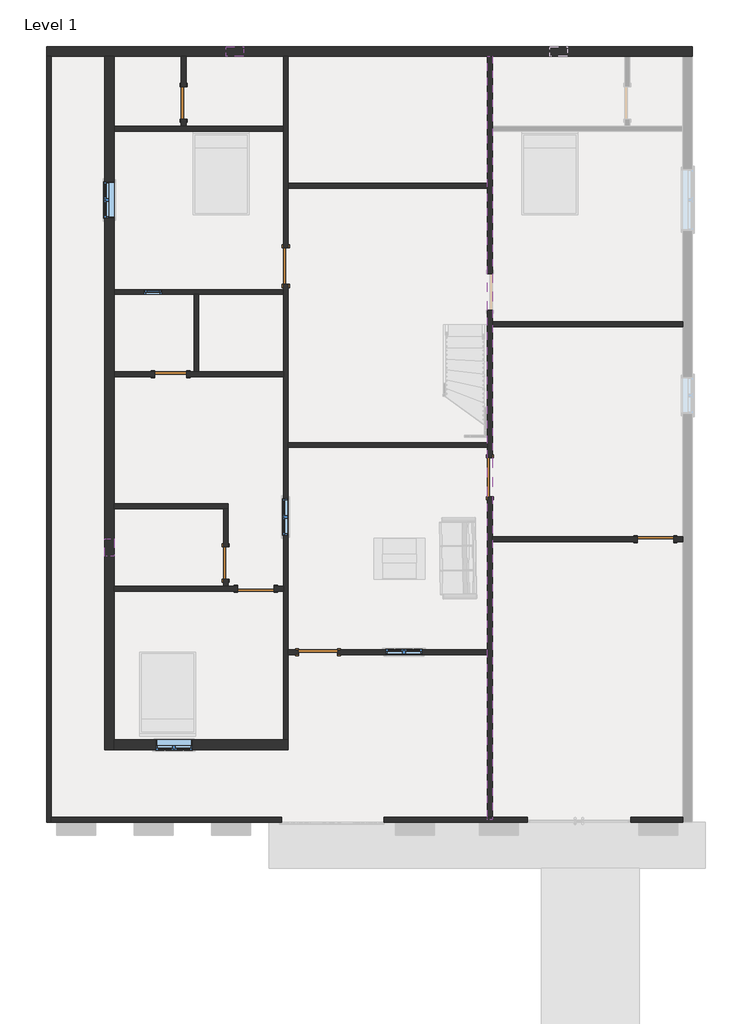
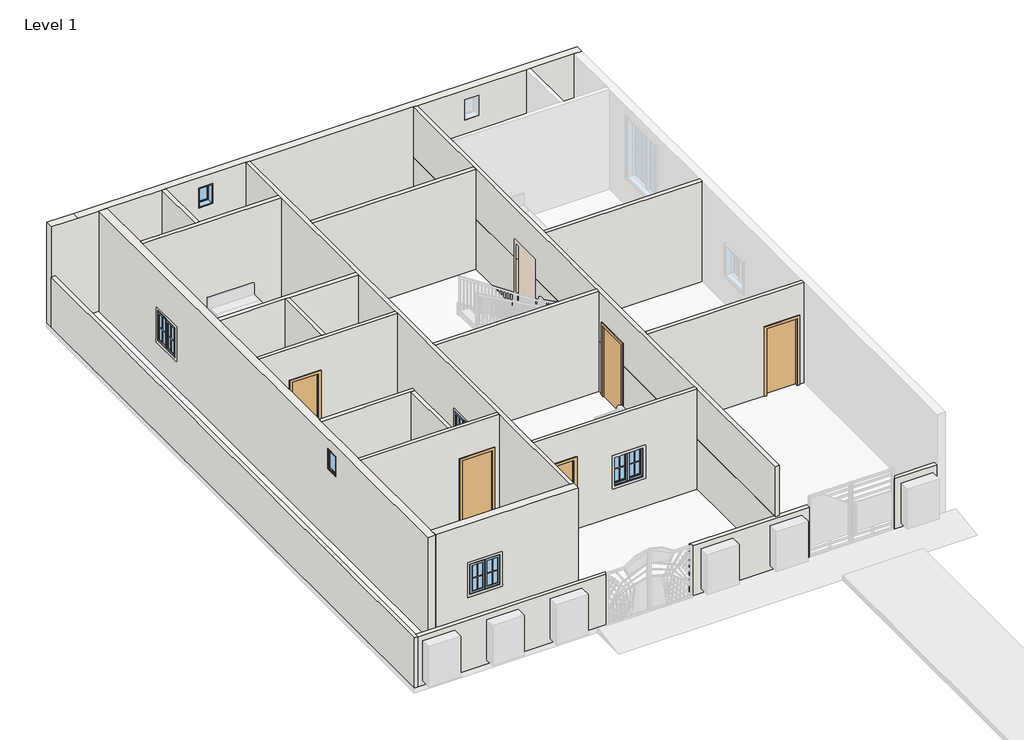
# One storey, part 1 of 3: 23 walls, 8 doors, 7 windows.
"""IFC4 building model written with IfcOpenShell, lengths in millimetres."""

from ifc_helpers import new_model, si_unit, frame, origin, origin_with_axes, place, context, project, spatial, polyline, outline, extrude, faceted_brep, transform, mapped, element, save
from components import door_f2b275c1, door_d8f5dbb5, door_825b8444, door_c29894e6, door_305aa2a5, window_aa618e30, window_a10b4202, window_339605e1, window_a598f463

model = new_model("IFC4")

# Units and contexts
model_context = context("Model", 3, world=origin())
ifc_project = project(units=[si_unit("LENGTHUNIT", "METRE", prefix="MILLI")], contexts=[model_context])

# Site, building, storey
site = spatial("IfcSite", under=ifc_project)
building = spatial("IfcBuilding", under=site)
storey = spatial("IfcBuildingStorey", under=building, Name="Level 1", Elevation=0.0)

# Doors
placement = place(None, origin())
door_shape = door_f2b275c1(model_context)
element("IfcDoor", 1, ObjectType="Single-Flush : 30\" x 80\"", at=placement, inside=storey, context=model_context, shape_type="MappedRepresentation", body=[
    mapped(door_shape, transform((-5639.8561469, 9100.7522623, 0.0), x_axis=(0.0, -1.0, 0.0), y_axis=(1.0, 0.0, 0.0), z_axis=(0.0, 0.0, 1.0))),
])
element("IfcDoor", 2, ObjectType="Single-Flush : 30\" x 80\"", at=placement, inside=storey, context=model_context, shape_type="MappedRepresentation", body=[
    mapped(door_shape, transform((-4646.033646, -1745.0477377, 0.0), x_axis=(0.0, -1.0, 0.0), y_axis=(1.0, 0.0, 0.0), z_axis=(0.0, 0.0, 1.0))),
])
door_2_shape = door_d8f5dbb5(model_context)
element("IfcDoor", 3, ObjectType="Single-Flush : 30\" x 80\"", at=placement, inside=storey, context=model_context, shape_type="MappedRepresentation", body=[
    mapped(door_2_shape, transform((-5947.8915084, 2699.9522623, 0.0), x_axis=(1.0, 0.0, 0.0), y_axis=(0.0, 1.0, 0.0), z_axis=(0.0, 0.0, 1.0))),
])
door_3_shape = door_825b8444(model_context)
element("IfcDoor", 4, ObjectType="Single-Flush : 34\" x 80\"", at=placement, inside=storey, context=model_context, shape_type="MappedRepresentation", body=[
    mapped(door_3_shape, transform((-3230.0915084, 5252.6522623, 0.0), x_axis=(0.0, -1.0, 0.0), y_axis=(1.0, 0.0, 0.0), z_axis=(0.0, 0.0, 1.0))),
])
element("IfcDoor", 5, ObjectType="Single-Flush : 34\" x 80\"", at=placement, inside=storey, context=model_context, shape_type="MappedRepresentation", body=[
    mapped(door_3_shape, transform((-3938.0625772, -2354.6477377, 0.0), x_axis=(1.0, 0.0, 0.0), y_axis=(0.0, 1.0, 0.0), z_axis=(0.0, 0.0, 1.0))),
])
door_4_shape = door_c29894e6(model_context)
element("IfcDoor", 6, ObjectType="Single-Flush : 34\" x 80\"", at=placement, inside=storey, context=model_context, shape_type="MappedRepresentation", body=[
    mapped(door_4_shape, transform((5488.4584916, -1186.2477377, 0.0), x_axis=(1.0, 0.0, 0.0), y_axis=(0.0, 1.0, 0.0), z_axis=(0.0, 0.0, 1.0))),
])
door_5_shape = door_305aa2a5(model_context)
element("IfcDoor", 7, ObjectType="Single-Flush : 36\" x 84\"", at=placement, inside=storey, context=model_context, shape_type="MappedRepresentation", body=[
    mapped(door_5_shape, transform((1583.2084916, 274.2522623, 0.0), x_axis=(0.0, -1.0, 0.0), y_axis=(1.0, 0.0, 0.0), z_axis=(0.0, 0.0, 1.0))),
])
element("IfcDoor", 8, ObjectType="Single-Flush : 36\" x 84\"", at=placement, inside=storey, context=model_context, shape_type="MappedRepresentation", body=[
    mapped(door_5_shape, transform((-2468.0915084, -3853.2477377, 0.0), x_axis=(-1.0, 0.0, 0.0), y_axis=(0.0, -1.0, 0.0), z_axis=(0.0, 0.0, 1.0))),
])

# Walls
element("IfcWall", 9, ObjectType="9\"", at=placement, inside=storey, context=model_context, shape_type="Brep", body=[
    faceted_brep([(-8875.2415084, 10199.3022623, 0.0), (-8760.9415084, 10199.3022623, 0.0), (-7503.6415084, 10199.3022623, 0.0), (-7275.0415084, 10199.3022623, 0.0), (-5697.0061469, 10199.3022623, 0.0), (-5582.7061469, 10199.3022623, 0.0), (-3287.2415084, 10199.3022623, 0.0), (-3172.9415084, 10199.3022623, 0.0), (1526.0584916, 10199.3022623, 0.0), (1640.3584916, 10199.3022623, 0.0), (4770.1866507, 10199.3022623, 0.0), (4884.4866507, 10199.3022623, 0.0), (6136.1584916, 10199.3022623, 0.0), (6364.7584916, 10199.3022623, 0.0), (6364.7584916, 10199.3022623, 3048.0), (6136.1584916, 10199.3022623, 3048.0), (4884.4866507, 10199.3022623, 3048.0), (4770.1866507, 10199.3022623, 3048.0), (1640.3584916, 10199.3022623, 3048.0), (1526.0584916, 10199.3022623, 3048.0), (-3172.9415084, 10199.3022623, 3048.0), (-3287.2415084, 10199.3022623, 3048.0), (-5582.7061469, 10199.3022623, 3048.0), (-5697.0061469, 10199.3022623, 3048.0), (-7275.0415084, 10199.3022623, 3048.0), (-7503.6415084, 10199.3022623, 3048.0), (-8113.2415084, 10199.3022623, 3048.0), (-8875.2415084, 10199.3022623, 3048.0), (-8875.2415084, 10199.3022623, 1524.0), (-4231.7738276, 10199.3022623, 2743.2), (-4231.7738276, 10199.3022623, 2133.6), (-4638.1738276, 10199.3022623, 2133.6), (-4638.1738276, 10199.3022623, 2743.2), (3408.4725711, 10199.3022623, 2743.2), (3408.4725711, 10199.3022623, 2133.6), (3002.0725711, 10199.3022623, 2133.6), (3002.0725711, 10199.3022623, 2743.2), (-8875.2415084, 10427.9022623, 0.0), (-8875.2415084, 10427.9022623, 3048.0), (-8113.2415084, 10427.9022623, 3048.0), (6364.7584916, 10427.9022623, 3048.0), (6364.7584916, 10427.9022623, 0.0), (-4231.7738276, 10427.9022623, 2743.2), (-4638.1738276, 10427.9022623, 2743.2), (-4638.1738276, 10427.9022623, 2133.6), (-4231.7738276, 10427.9022623, 2133.6), (3408.4725711, 10427.9022623, 2743.2), (3002.0725711, 10427.9022623, 2743.2), (3002.0725711, 10427.9022623, 2133.6), (3408.4725711, 10427.9022623, 2133.6)], [[[0, 1, 2, 3, 4, 5, 6, 7, 8, 9, 10, 11, 12, 13, 14, 15, 16, 17, 18, 19, 20, 21, 22, 23, 24, 25, 26, 27, 28], [29, 30, 31, 32], [33, 34, 35, 36]], [[37, 38, 39, 40, 41], [42, 43, 44, 45], [46, 47, 48, 49]], [[13, 12, 11, 10, 9, 8, 7, 6, 5, 4, 3, 2, 1, 0, 37, 41]], [[14, 13, 41, 40]], [[0, 28, 27, 38, 37]], [[30, 29, 42, 45]], [[31, 30, 45, 44]], [[32, 31, 44, 43]], [[29, 32, 43, 42]], [[34, 33, 46, 49]], [[35, 34, 49, 48]], [[36, 35, 48, 47]], [[33, 36, 47, 46]], [[27, 26, 39, 38]], [[26, 25, 24, 23, 22, 21, 20, 19, 18, 17, 16, 15, 14, 40, 39]]]),
])
element("IfcWall", 10, ObjectType="9\"", at=placement, inside=storey, context=model_context, shape_type="Brep", body=[
    faceted_brep([(-7503.6415084, 10199.3022623, 0.0), (-7503.6415084, -6145.5977377, 0.0), (-7503.6415084, -6145.5977377, 3048.0), (-7503.6415084, 10199.3022623, 3048.0), (-7503.6415084, -1179.8977377, 2743.2), (-7503.6415084, -1586.2977377, 2743.2), (-7503.6415084, -1586.2977377, 2133.6), (-7503.6415084, -1179.8977377, 2133.6), (-7503.6415084, 7246.5522623, 1828.8), (-7503.6415084, 6382.9522623, 1828.8), (-7503.6415084, 6382.9522623, 914.4), (-7503.6415084, 7246.5522623, 914.4), (-7275.0415084, 10199.3022623, 0.0), (-7275.0415084, 10199.3022623, 3048.0), (-7275.0415084, 8548.3022623, 3048.0), (-7275.0415084, 8434.0022623, 3048.0), (-7275.0415084, 4700.2022623, 3048.0), (-7275.0415084, 4585.9022623, 3048.0), (-7275.0415084, 2757.1022623, 3048.0), (-7275.0415084, 2642.8022623, 3048.0), (-7275.0415084, -354.3977377, 3048.0), (-7275.0415084, -468.6977377, 3048.0), (-7275.0415084, -2297.4977377, 3048.0), (-7275.0415084, -2411.7977377, 3048.0), (-7275.0415084, -5916.9977377, 3048.0), (-7275.0415084, -6145.5977377, 3048.0), (-7275.0415084, -6145.5977377, 0.0), (-7275.0415084, -5916.9977377, 0.0), (-7275.0415084, -2411.7977377, 0.0), (-7275.0415084, -2297.4977377, 0.0), (-7275.0415084, -468.6977377, 0.0), (-7275.0415084, -354.3977377, 0.0), (-7275.0415084, 2642.8022623, 0.0), (-7275.0415084, 2757.1022623, 0.0), (-7275.0415084, 4585.9022623, 0.0), (-7275.0415084, 4700.2022623, 0.0), (-7275.0415084, 8434.0022623, 0.0), (-7275.0415084, 8548.3022623, 0.0), (-7275.0415084, -1179.8977377, 2743.2), (-7275.0415084, -1179.8977377, 2133.6), (-7275.0415084, -1586.2977377, 2133.6), (-7275.0415084, -1586.2977377, 2743.2), (-7275.0415084, 7246.5522623, 1828.8), (-7275.0415084, 7246.5522623, 914.4), (-7275.0415084, 6382.9522623, 914.4), (-7275.0415084, 6382.9522623, 1828.8)], [[[0, 1, 2, 3], [4, 5, 6, 7], [8, 9, 10, 11]], [[12, 13, 14, 15, 16, 17, 18, 19, 20, 21, 22, 23, 24, 25, 26, 27, 28, 29, 30, 31, 32, 33, 34, 35, 36, 37], [38, 39, 40, 41], [42, 43, 44, 45]], [[1, 0, 12, 37, 36, 35, 34, 33, 32, 31, 30, 29, 28, 27, 26]], [[0, 3, 13, 12]], [[2, 1, 26, 25]], [[39, 38, 4, 7]], [[40, 39, 7, 6]], [[41, 40, 6, 5]], [[38, 41, 5, 4]], [[43, 42, 8, 11]], [[44, 43, 11, 10]], [[45, 44, 10, 9]], [[42, 45, 9, 8]], [[3, 2, 25, 24, 23, 22, 21, 20, 19, 18, 17, 16, 15, 14, 13]]]),
])
element("IfcWall", 11, ObjectType="9\"", at=placement, inside=storey, context=model_context, shape_type="Brep", body=[
    faceted_brep([(-7275.0415084, -6145.5977377, 0.0), (-3172.9415084, -6145.5977377, 0.0), (-3172.9415084, -6145.5977377, 3048.0), (-7275.0415084, -6145.5977377, 3048.0), (-6297.1415084, -6145.5977377, 1828.8), (-5433.5415084, -6145.5977377, 1828.8), (-5433.5415084, -6145.5977377, 914.4), (-6297.1415084, -6145.5977377, 914.4), (-7275.0415084, -5916.9977377, 0.0), (-7275.0415084, -5916.9977377, 3048.0), (-3287.2415084, -5916.9977377, 3048.0), (-3172.9415084, -5916.9977377, 3048.0), (-3172.9415084, -5916.9977377, 0.0), (-3287.2415084, -5916.9977377, 0.0), (-6297.1415084, -5916.9977377, 1828.8), (-6297.1415084, -5916.9977377, 914.4), (-5433.5415084, -5916.9977377, 914.4), (-5433.5415084, -5916.9977377, 1828.8)], [[[0, 1, 2, 3], [4, 5, 6, 7]], [[8, 9, 10, 11, 12, 13], [14, 15, 16, 17]], [[1, 0, 8, 13, 12]], [[0, 3, 9, 8]], [[2, 1, 12, 11]], [[15, 14, 4, 7]], [[16, 15, 7, 6]], [[17, 16, 6, 5]], [[14, 17, 5, 4]], [[3, 2, 11, 10, 9]]]),
])
element("IfcWall", 12, ObjectType="WALL4.5\"", at=placement, inside=storey, context=model_context, shape_type="Brep", body=[
    faceted_brep([(-8875.2415084, 10199.3022623, 0.0), (-8875.2415084, -7860.0977377, 0.0), (-8875.2415084, -7860.0977377, 1524.0), (-8875.2415084, 10199.3022623, 1524.0), (-8760.9415084, 10199.3022623, 0.0), (-8760.9415084, 10199.3022623, 1524.0), (-8760.9415084, -7745.7977377, 1524.0), (-8760.9415084, -7860.0977377, 1524.0), (-8760.9415084, -7860.0977377, 0.0), (-8760.9415084, -7745.7977377, 0.0)], [[[0, 1, 2, 3]], [[4, 5, 6, 7, 8, 9]], [[1, 0, 4, 9, 8]], [[3, 2, 7, 6, 5]], [[0, 3, 5, 4]], [[2, 1, 8, 7]]]),
])
element("IfcWall", 13, ObjectType="WALL4.5\"", at=placement, inside=storey, context=model_context, shape_type="SweptSolid", body=[
    extrude(outline(polyline([(-3331.6915084, -7860.0977377), (-8760.9415084, -7860.0977377), (-8760.9415084, -7745.7977377), (-3331.6915084, -7745.7977377), (-3331.6915084, -7860.0977377)])), origin_with_axes(), (0.0, 0.0, 1.0), 1524.0),
])
element("IfcWall", 14, ObjectType="WALL4.5\"", at=placement, inside=storey, context=model_context, shape_type="Brep", body=[
    faceted_brep([(-7275.0415084, 8434.0022623, 0.0), (-3287.2415084, 8434.0022623, 0.0), (-3287.2415084, 8434.0022623, 3048.0), (-7275.0415084, 8434.0022623, 3048.0), (-7275.0415084, 8548.3022623, 0.0), (-7275.0415084, 8548.3022623, 3048.0), (-5697.0061469, 8548.3022623, 3048.0), (-5582.7061469, 8548.3022623, 3048.0), (-3287.2415084, 8548.3022623, 3048.0), (-3287.2415084, 8548.3022623, 0.0), (-5582.7061469, 8548.3022623, 0.0), (-5697.0061469, 8548.3022623, 0.0)], [[[0, 1, 2, 3]], [[4, 5, 6, 7, 8, 9, 10, 11]], [[1, 0, 4, 11, 10, 9]], [[0, 3, 5, 4]], [[2, 1, 9, 8]], [[3, 2, 8, 7, 6, 5]]]),
])
element("IfcWall", 15, ObjectType="WALL4.5\"", at=placement, inside=storey, context=model_context, shape_type="SweptSolid", body=[
    extrude(outline(polyline([(8719.7522623, 2032.0), (8719.7522623, 0.0), (8548.3022623, 0.0), (8548.3022623, 3048.0), (10199.3022623, 3048.0), (10199.3022623, 0.0), (9481.7522623, 0.0), (9481.7522623, 2032.0), (8719.7522623, 2032.0)])), frame((-5697.0061469, 0.0, 0.0), z_axis=(1.0, 0.0, 0.0), x_axis=(0.0, 1.0, 0.0)), (0.0, 0.0, 1.0), 114.3),
])
element("IfcWall", 16, ObjectType="WALL4.5\"", at=placement, inside=storey, context=model_context, shape_type="Brep", body=[
    faceted_brep([(-3287.2415084, 4820.8522623, 2032.0), (-3287.2415084, 4820.8522623, 0.0), (-3287.2415084, 4700.2022623, 0.0), (-3287.2415084, 4585.9022623, 0.0), (-3287.2415084, 2757.1022623, 0.0), (-3287.2415084, 2642.8022623, 0.0), (-3287.2415084, -2297.4977377, 0.0), (-3287.2415084, -2411.7977377, 0.0), (-3287.2415084, -5916.9977377, 0.0), (-3287.2415084, -5916.9977377, 3048.0), (-3287.2415084, -2411.7977377, 3048.0), (-3287.2415084, -2297.4977377, 3048.0), (-3287.2415084, 2642.8022623, 3048.0), (-3287.2415084, 2757.1022623, 3048.0), (-3287.2415084, 4585.9022623, 3048.0), (-3287.2415084, 4700.2022623, 3048.0), (-3287.2415084, 8434.0022623, 3048.0), (-3287.2415084, 8548.3022623, 3048.0), (-3287.2415084, 10199.3022623, 3048.0), (-3287.2415084, 10199.3022623, 0.0), (-3287.2415084, 8548.3022623, 0.0), (-3287.2415084, 8434.0022623, 0.0), (-3287.2415084, 5684.4522623, 0.0), (-3287.2415084, 5684.4522623, 2032.0), (-3287.2415084, -227.3977377, 1828.8), (-3287.2415084, -1090.9977377, 1828.8), (-3287.2415084, -1090.9977377, 914.4), (-3287.2415084, -227.3977377, 914.4), (-3172.9415084, -5916.9977377, 0.0), (-3172.9415084, -3910.3977377, 0.0), (-3172.9415084, -3796.0977377, 0.0), (-3172.9415084, 979.1022623, 0.0), (-3172.9415084, 1093.4022623, 0.0), (-3172.9415084, 4820.8522623, 0.0), (-3172.9415084, 4820.8522623, 2032.0), (-3172.9415084, 5684.4522623, 2032.0), (-3172.9415084, 5684.4522623, 0.0), (-3172.9415084, 7087.8022623, 0.0), (-3172.9415084, 7202.1022623, 0.0), (-3172.9415084, 10199.3022623, 0.0), (-3172.9415084, 10199.3022623, 3048.0), (-3172.9415084, 7202.1022623, 3048.0), (-3172.9415084, 7087.8022623, 3048.0), (-3172.9415084, 1093.4022623, 3048.0), (-3172.9415084, 979.1022623, 3048.0), (-3172.9415084, -3796.0977377, 3048.0), (-3172.9415084, -3910.3977377, 3048.0), (-3172.9415084, -5916.9977377, 3048.0), (-3172.9415084, -227.3977377, 1828.8), (-3172.9415084, -227.3977377, 914.4), (-3172.9415084, -1090.9977377, 914.4), (-3172.9415084, -1090.9977377, 1828.8)], [[[0, 1, 2, 3, 4, 5, 6, 7, 8, 9, 10, 11, 12, 13, 14, 15, 16, 17, 18, 19, 20, 21, 22, 23], [24, 25, 26, 27]], [[28, 29, 30, 31, 32, 33, 34, 35, 36, 37, 38, 39, 40, 41, 42, 43, 44, 45, 46, 47], [48, 49, 50, 51]], [[22, 21, 20, 19, 39, 38, 37, 36]], [[8, 7, 6, 5, 4, 3, 2, 1, 33, 32, 31, 30, 29, 28]], [[9, 8, 28, 47]], [[19, 18, 40, 39]], [[34, 33, 1, 0]], [[35, 34, 0, 23]], [[36, 35, 23, 22]], [[49, 48, 24, 27]], [[50, 49, 27, 26]], [[51, 50, 26, 25]], [[48, 51, 25, 24]], [[18, 17, 16, 15, 14, 13, 12, 11, 10, 9, 47, 46, 45, 44, 43, 42, 41, 40]]]),
])
element("IfcWall", 17, ObjectType="WALL4.5\"", at=placement, inside=storey, context=model_context, shape_type="Brep", body=[
    faceted_brep([(-7275.0415084, 4585.9022623, 0.0), (-5395.4415084, 4585.9022623, 0.0), (-5281.1415084, 4585.9022623, 0.0), (-3287.2415084, 4585.9022623, 0.0), (-3287.2415084, 4585.9022623, 3048.0), (-5281.1415084, 4585.9022623, 3048.0), (-5395.4415084, 4585.9022623, 3048.0), (-7275.0415084, 4585.9022623, 3048.0), (-6160.6165084, 4585.9022623, 1524.0), (-6160.6165084, 4585.9022623, 914.4), (-6567.0165084, 4585.9022623, 914.4), (-6567.0165084, 4585.9022623, 1524.0), (-7275.0415084, 4700.2022623, 0.0), (-7275.0415084, 4700.2022623, 3048.0), (-3287.2415084, 4700.2022623, 3048.0), (-3287.2415084, 4700.2022623, 0.0), (-6160.6165084, 4700.2022623, 1524.0), (-6567.0165084, 4700.2022623, 1524.0), (-6567.0165084, 4700.2022623, 914.4), (-6160.6165084, 4700.2022623, 914.4)], [[[0, 1, 2, 3, 4, 5, 6, 7], [8, 9, 10, 11]], [[12, 13, 14, 15], [16, 17, 18, 19]], [[3, 2, 1, 0, 12, 15]], [[0, 7, 13, 12]], [[4, 3, 15, 14]], [[9, 8, 16, 19]], [[10, 9, 19, 18]], [[11, 10, 18, 17]], [[8, 11, 17, 16]], [[7, 6, 5, 4, 14, 13]]]),
])
element("IfcWall", 18, ObjectType="WALL4.5\"", at=placement, inside=storey, context=model_context, shape_type="SweptSolid", body=[
    extrude(outline(polyline([(-5395.4415084, 2757.1022623), (-5395.4415084, 4585.9022623), (-5281.1415084, 4585.9022623), (-5281.1415084, 2757.1022623), (-5395.4415084, 2757.1022623)])), origin_with_axes(), (0.0, 0.0, 1.0), 3048.0),
])
element("IfcWall", 19, ObjectType="WALL4.5\"", at=placement, inside=storey, context=model_context, shape_type="Brep", body=[
    faceted_brep([(-5566.8915084, 2642.8022623, 2032.0), (-5566.8915084, 2642.8022623, 0.0), (-3287.2415084, 2642.8022623, 0.0), (-3287.2415084, 2642.8022623, 3048.0), (-7275.0415084, 2642.8022623, 3048.0), (-7275.0415084, 2642.8022623, 0.0), (-6328.8915084, 2642.8022623, 0.0), (-6328.8915084, 2642.8022623, 2032.0), (-3287.2415084, 2757.1022623, 0.0), (-5281.1415084, 2757.1022623, 0.0), (-5395.4415084, 2757.1022623, 0.0), (-5566.8915084, 2757.1022623, 0.0), (-5566.8915084, 2757.1022623, 2032.0), (-6328.8915084, 2757.1022623, 2032.0), (-6328.8915084, 2757.1022623, 0.0), (-7275.0415084, 2757.1022623, 0.0), (-7275.0415084, 2757.1022623, 3048.0), (-5395.4415084, 2757.1022623, 3048.0), (-5281.1415084, 2757.1022623, 3048.0), (-3287.2415084, 2757.1022623, 3048.0)], [[[0, 1, 2, 3, 4, 5, 6, 7]], [[8, 9, 10, 11, 12, 13, 14, 15, 16, 17, 18, 19]], [[6, 5, 15, 14]], [[2, 1, 11, 10, 9, 8]], [[5, 4, 16, 15]], [[3, 2, 8, 19]], [[12, 11, 1, 0]], [[13, 12, 0, 7]], [[14, 13, 7, 6]], [[4, 3, 19, 18, 17, 16]]]),
])
element("IfcWall", 20, ObjectType="WALL4.5\"", at=placement, inside=storey, context=model_context, shape_type="Brep", body=[
    faceted_brep([(-7275.0415084, -468.6977377, 0.0), (-4703.183646, -468.6977377, 0.0), (-4588.883646, -468.6977377, 0.0), (-4588.883646, -468.6977377, 3048.0), (-4703.183646, -468.6977377, 3048.0), (-7275.0415084, -468.6977377, 3048.0), (-7275.0415084, -354.3977377, 0.0), (-7275.0415084, -354.3977377, 3048.0), (-4588.883646, -354.3977377, 3048.0), (-4588.883646, -354.3977377, 0.0)], [[[0, 1, 2, 3, 4, 5]], [[6, 7, 8, 9]], [[2, 1, 0, 6, 9]], [[0, 5, 7, 6]], [[3, 2, 9, 8]], [[5, 4, 3, 8, 7]]]),
])
element("IfcWall", 21, ObjectType="WALL4.5\"", at=placement, inside=storey, context=model_context, shape_type="SweptSolid", body=[
    extrude(outline(polyline([(-2126.0477377, 2032.0), (-2126.0477377, 0.0), (-2297.4977377, 0.0), (-2297.4977377, 3048.0), (-468.6977377, 3048.0), (-468.6977377, 0.0), (-1364.0477377, 0.0), (-1364.0477377, 2032.0), (-2126.0477377, 2032.0)])), frame((-4703.183646, 0.0, 0.0), z_axis=(1.0, 0.0, 0.0), x_axis=(0.0, 1.0, 0.0)), (0.0, 0.0, 1.0), 114.3),
])
element("IfcWall", 22, ObjectType="WALL4.5\"", at=placement, inside=storey, context=model_context, shape_type="Brep", body=[
    faceted_brep([(-3506.2625772, -2411.7977377, 2032.0), (-3506.2625772, -2411.7977377, 0.0), (-3287.2415084, -2411.7977377, 0.0), (-3287.2415084, -2411.7977377, 3048.0), (-7275.0415084, -2411.7977377, 3048.0), (-7275.0415084, -2411.7977377, 0.0), (-4369.8625772, -2411.7977377, 0.0), (-4369.8625772, -2411.7977377, 2032.0), (-3287.2415084, -2297.4977377, 0.0), (-3506.2625772, -2297.4977377, 0.0), (-3506.2625772, -2297.4977377, 2032.0), (-4369.8625772, -2297.4977377, 2032.0), (-4369.8625772, -2297.4977377, 0.0), (-4588.883646, -2297.4977377, 0.0), (-4703.183646, -2297.4977377, 0.0), (-7275.0415084, -2297.4977377, 0.0), (-7275.0415084, -2297.4977377, 3048.0), (-4703.183646, -2297.4977377, 3048.0), (-4588.883646, -2297.4977377, 3048.0), (-3287.2415084, -2297.4977377, 3048.0)], [[[0, 1, 2, 3, 4, 5, 6, 7]], [[8, 9, 10, 11, 12, 13, 14, 15, 16, 17, 18, 19]], [[6, 5, 15, 14, 13, 12]], [[2, 1, 9, 8]], [[5, 4, 16, 15]], [[3, 2, 8, 19]], [[10, 9, 1, 0]], [[11, 10, 0, 7]], [[12, 11, 7, 6]], [[4, 3, 19, 18, 17, 16]]]),
])
element("IfcWall", 23, ObjectType="WALL4.5\"", at=placement, inside=storey, context=model_context, shape_type="SweptSolid", body=[
    extrude(outline(polyline([(1526.0584916, 7087.8022623), (-3172.9415084, 7087.8022623), (-3172.9415084, 7202.1022623), (1526.0584916, 7202.1022623), (1526.0584916, 7087.8022623)])), origin_with_axes(), (0.0, 0.0, 1.0), 3048.0),
])
element("IfcWall", 24, ObjectType="WALL4.5\"", at=placement, inside=storey, context=model_context, shape_type="Brep", body=[
    faceted_brep([(1526.0584916, 10199.3022623, 1524.0), (1526.0584916, 10199.3022623, 0.0), (1526.0584916, 7202.1022623, 0.0), (1526.0584916, 7087.8022623, 0.0), (1526.0584916, 5074.8522623, 0.0), (1526.0584916, 5074.8522623, 1524.0), (1640.3584916, 10199.3022623, 0.0), (1640.3584916, 10199.3022623, 1524.0), (1640.3584916, 5074.8522623, 1524.0), (1640.3584916, 5074.8522623, 0.0), (1640.3584916, 8434.0022623, 0.0), (1640.3584916, 8548.3022623, 0.0)], [[[0, 1, 2, 3, 4, 5]], [[6, 7, 8, 9, 10, 11]], [[1, 6, 11, 10, 9, 4, 3, 2]], [[7, 0, 5, 8]], [[1, 0, 7, 6]], [[5, 4, 9, 8]]]),
    faceted_brep([(1526.0584916, -7745.7977377, 0.0), (1526.0584916, -7745.7977377, 1524.0), (1526.0584916, -182.9477377, 1524.0), (1526.0584916, -182.9477377, 0.0), (1526.0584916, -3796.0977377, 0.0), (1526.0584916, -3910.3977377, 0.0), (1640.3584916, -7745.7977377, 1524.0), (1640.3584916, -7745.7977377, 0.0), (1640.3584916, -1243.3977377, 0.0), (1640.3584916, -1129.0977377, 0.0), (1640.3584916, -182.9477377, 0.0), (1640.3584916, -182.9477377, 1524.0)], [[[0, 1, 2, 3, 4, 5]], [[6, 7, 8, 9, 10, 11]], [[7, 0, 5, 4, 3, 10, 9, 8]], [[1, 6, 11, 2]], [[1, 0, 7, 6]], [[3, 2, 11, 10]]]),
    faceted_brep([(1526.0584916, 4211.2522623, 1524.0), (1526.0584916, 4211.2522623, 0.0), (1526.0584916, 1093.4022623, 0.0), (1526.0584916, 979.1022623, 0.0), (1526.0584916, 731.4522623, 0.0), (1526.0584916, 731.4522623, 1524.0), (1640.3584916, 4211.2522623, 0.0), (1640.3584916, 4211.2522623, 1524.0), (1640.3584916, 731.4522623, 1524.0), (1640.3584916, 731.4522623, 0.0), (1640.3584916, 3823.9022623, 0.0), (1640.3584916, 3938.2022623, 0.0)], [[[0, 1, 2, 3, 4, 5]], [[6, 7, 8, 9, 10, 11]], [[1, 6, 11, 10, 9, 4, 3, 2]], [[7, 0, 5, 8]], [[1, 0, 7, 6]], [[5, 4, 9, 8]]]),
])
element("IfcWall", 25, ObjectType="WALL4.5\"", at=placement, inside=storey, context=model_context, shape_type="SweptSolid", body=[
    extrude(outline(polyline([(0.0, -3172.9415084), (0.0, -2925.2915084), (2133.6, -2925.2915084), (2133.6, -2010.8915084), (0.0, -2010.8915084), (0.0, 1526.0584916), (3048.0, 1526.0584916), (3048.0, -3172.9415084), (0.0, -3172.9415084)]), holes=[polyline([(1828.8, -10.6415084), (914.4, -10.6415084), (914.4, -874.2415084), (1828.8, -874.2415084), (1828.8, -10.6415084)])]), frame((0.0, -3910.3977377, 0.0), z_axis=(0.0, 1.0, 0.0), x_axis=(0.0, 0.0, 1.0)), (0.0, 0.0, 1.0), 114.3),
])
element("IfcWall", 26, ObjectType="WALL4.5\"", at=placement, inside=storey, context=model_context, shape_type="SweptSolid", body=[
    extrude(outline(polyline([(1526.0584916, 979.1022623), (-3172.9415084, 979.1022623), (-3172.9415084, 1093.4022623), (1526.0584916, 1093.4022623), (1526.0584916, 979.1022623)])), origin_with_axes(), (0.0, 0.0, 1.0), 3048.0),
])
element("IfcWall", 27, ObjectType="WALL4.5\"", at=placement, inside=storey, context=model_context, shape_type="SweptSolid", body=[
    extrude(outline(polyline([(6136.1584916, 3823.9022623), (1640.3584916, 3823.9022623), (1640.3584916, 3938.2022623), (6136.1584916, 3938.2022623), (6136.1584916, 3823.9022623)])), origin_with_axes(), (0.0, 0.0, 1.0), 3048.0),
])
element("IfcWall", 28, ObjectType="WALL4.5\"", at=placement, inside=storey, context=model_context, shape_type="SweptSolid", body=[
    extrude(outline(polyline([(2032.0, 5920.2584916), (0.0, 5920.2584916), (0.0, 6136.1584916), (3048.0, 6136.1584916), (3048.0, 1640.3584916), (0.0, 1640.3584916), (0.0, 5056.6584916), (2032.0, 5056.6584916), (2032.0, 5920.2584916)])), frame((0.0, -1243.3977377, 0.0), z_axis=(0.0, 1.0, 0.0), x_axis=(0.0, 0.0, 1.0)), (0.0, 0.0, 1.0), 114.3),
])
element("IfcWall", 29, ObjectType="WALL4.5\"", at=placement, inside=storey, context=model_context, shape_type="Brep", body=[
    faceted_brep([(1526.0584916, -7802.9477377, 1524.0), (1526.0584916, -7802.9477377, 3048.0), (1526.0584916, 10199.3022623, 3048.0), (1526.0584916, 10199.3022623, 1524.0), (1526.0584916, 5074.8522623, 1524.0), (1526.0584916, 5074.8522623, 2032.0), (1526.0584916, 4211.2522623, 2032.0), (1526.0584916, 4211.2522623, 1524.0), (1526.0584916, 731.4522623, 1524.0), (1526.0584916, 731.4522623, 2133.6), (1526.0584916, -182.9477377, 2133.6), (1526.0584916, -182.9477377, 1524.0), (1526.0584916, -7745.7977377, 1524.0), (1640.3584916, -7802.9477377, 3048.0), (1640.3584916, -7802.9477377, 1524.0), (1640.3584916, -7745.7977377, 1524.0), (1640.3584916, -182.9477377, 1524.0), (1640.3584916, -182.9477377, 2133.6), (1640.3584916, 731.4522623, 2133.6), (1640.3584916, 731.4522623, 1524.0), (1640.3584916, 4211.2522623, 1524.0), (1640.3584916, 4211.2522623, 2032.0), (1640.3584916, 5074.8522623, 2032.0), (1640.3584916, 5074.8522623, 1524.0), (1640.3584916, 10199.3022623, 1524.0), (1640.3584916, 10199.3022623, 3048.0)], [[[0, 1, 2, 3, 4, 5, 6, 7, 8, 9, 10, 11, 12]], [[13, 14, 15, 16, 17, 18, 19, 20, 21, 22, 23, 24, 25]], [[14, 0, 12, 11, 16, 15]], [[7, 20, 19, 8]], [[4, 3, 24, 23]], [[1, 0, 14, 13]], [[6, 21, 20, 7]], [[21, 6, 5, 22]], [[22, 5, 4, 23]], [[10, 17, 16, 11]], [[17, 10, 9, 18]], [[18, 9, 8, 19]], [[3, 2, 25, 24]], [[2, 1, 13, 25]]]),
])
element("IfcWall", 30, ObjectType="WALL4.5\"", at=placement, inside=storey, context=model_context, shape_type="SweptSolid", body=[
    extrude(outline(polyline([(6136.1584916, -7860.0977377), (4904.2584916, -7860.0977377), (4904.2584916, -7745.7977377), (6136.1584916, -7745.7977377), (6136.1584916, -7860.0977377)])), origin_with_axes(), (0.0, 0.0, 1.0), 1524.0),
])
element("IfcWall", 31, ObjectType="WALL4.5\"", at=placement, inside=storey, context=model_context, shape_type="Brep", body=[
    faceted_brep([(-916.1049597, -7860.0977377, 0.0), (2465.8584916, -7860.0977377, 0.0), (2465.8584916, -7860.0977377, 1524.0), (-916.1049597, -7860.0977377, 1524.0), (-916.1049597, -7745.7977377, 0.0), (-916.1049597, -7745.7977377, 1524.0), (1526.0584916, -7745.7977377, 1524.0), (1640.3584916, -7745.7977377, 1524.0), (2465.8584916, -7745.7977377, 1524.0), (2465.8584916, -7745.7977377, 0.0), (1640.3584916, -7745.7977377, 0.0), (1526.0584916, -7745.7977377, 0.0)], [[[0, 1, 2, 3]], [[4, 5, 6, 7, 8, 9, 10, 11]], [[1, 0, 4, 11, 10, 9]], [[2, 1, 9, 8]], [[3, 2, 8, 7, 6, 5]], [[0, 3, 5, 4]]]),
])

# Windows
window_shape = window_aa618e30(model_context)
element("IfcWindow", 32, ObjectType="Fixed : 16\" x 24\"", at=placement, inside=storey, context=model_context, shape_type="MappedRepresentation", body=[
    mapped(window_shape, transform((-4396.8738276, 10313.6022623, 1219.2), x_axis=(1.0, 0.0, 0.0), y_axis=(0.0, 1.0, 0.0), z_axis=(0.0, 0.0, 1.0))),
])
element("IfcWindow", 33, ObjectType="Fixed : 16\" x 24\"", at=placement, inside=storey, context=model_context, shape_type="MappedRepresentation", body=[
    mapped(window_shape, transform((-7389.3415084, -1344.9977377, 1219.2), x_axis=(0.0, 1.0, 0.0), y_axis=(-1.0, 0.0, 0.0), z_axis=(0.0, 0.0, 1.0))),
])
window_2_shape = window_a10b4202(model_context)
element("IfcWindow", 34, ObjectType="Fixed : 16\" x 24\"", at=placement, inside=storey, context=model_context, shape_type="MappedRepresentation", body=[
    mapped(window_2_shape, transform((-6325.7165084, 4643.0522623, 0.0), x_axis=(1.0, 0.0, 0.0), y_axis=(0.0, 1.0, 0.0), z_axis=(0.0, 0.0, 1.0))),
])
window_3_shape = window_339605e1(model_context)
element("IfcWindow", 35, ObjectType="Window-Casement-Double : 34\" x 36\"", at=placement, inside=storey, context=model_context, shape_type="MappedRepresentation", body=[
    mapped(window_3_shape, transform((-7389.3415084, 6814.7522623, 0.0), x_axis=(0.0, 1.0, 0.0), y_axis=(-1.0, 0.0, 0.0), z_axis=(0.0, 0.0, 1.0))),
])
element("IfcWindow", 36, ObjectType="Window-Casement-Double : 34\" x 36\"", at=placement, inside=storey, context=model_context, shape_type="MappedRepresentation", body=[
    mapped(window_3_shape, transform((-5865.3415084, -6031.2977377, 0.0), x_axis=(-1.0, 0.0, 0.0), y_axis=(0.0, -1.0, 0.0), z_axis=(0.0, 0.0, 1.0))),
])
window_4_shape = window_a598f463(model_context)
element("IfcWindow", 37, ObjectType="Window-Casement-Double : 34\" x 36\"", at=placement, inside=storey, context=model_context, shape_type="MappedRepresentation", body=[
    mapped(window_4_shape, transform((-442.4415084, -3853.2477377, 0.0), x_axis=(1.0, 0.0, 0.0), y_axis=(0.0, 1.0, 0.0), z_axis=(0.0, 0.0, 1.0))),
])
element("IfcWindow", 38, ObjectType="Window-Casement-Double : 34\" x 36\"", at=placement, inside=storey, context=model_context, shape_type="MappedRepresentation", body=[
    mapped(window_4_shape, transform((-3230.0915084, -659.1977377, 0.0), x_axis=(0.0, 1.0, 0.0), y_axis=(-1.0, 0.0, 0.0), z_axis=(0.0, 0.0, 1.0))),
])

save(model, "model.ifc")

# Revit data of these elements
# Type "Single-Flush : 30\" x 80\""
#   Type Mark = "5"
#   Construction Type Id = "MDOOR"
#   Assembly Code = "C1020"
#   Analytic Construction = "Metal"
#   Thickness = 0' - 2"
#   Heat Transfer Coefficient (U) = 0.651978 BTU/(h·ft²·°F)
#   Height = 6' - 8"
#   Trim Projection Ext = 0' - 1"
#   Trim Projection Int = 0' - 1"
#   Trim Width = 0' - 3"
#   Width = 2' - 6"
#   Define Thermal Properties by = 1
#   Define Thermal Properties by = 1
#   Door Material = Door - Panel
#   Frame Material = Door - Frame
#   Visual Light Transmittance = 0
#   Solar Heat Gain Coefficient = 0
#   Function = (empty or 0)
#   Wall Closure = (empty or 0)
# Type "Single-Flush : 34\" x 80\""
#   Type Mark = "7"
#   Construction Type Id = "MDOOR"
#   Assembly Code = "C1020"
#   Analytic Construction = "Metal"
#   Thickness = 0' - 2"
#   Heat Transfer Coefficient (U) = 0.651978 BTU/(h·ft²·°F)
#   Height = 6' - 8"
#   Trim Projection Ext = 0' - 1"
#   Trim Projection Int = 0' - 1"
#   Trim Width = 0' - 3"
#   Width = 2' - 10"
#   Define Thermal Properties by = 1
#   Define Thermal Properties by = 1
#   Door Material = Door - Panel
#   Frame Material = Door - Frame
#   Visual Light Transmittance = 0
#   Solar Heat Gain Coefficient = 0
#   Function = (empty or 0)
#   Wall Closure = (empty or 0)
# Type "Single-Flush : 36\" x 84\""
#   Type Mark = "1"
#   Construction Type Id = "MDOOR"
#   Assembly Code = "C1020"
#   Analytic Construction = "Metal"
#   Thickness = 0' - 2"
#   Heat Transfer Coefficient (U) = 0.651978 BTU/(h·ft²·°F)
#   Height = 7' - 0"
#   Trim Projection Ext = 0' - 1"
#   Trim Projection Int = 0' - 1"
#   Trim Width = 0' - 3"
#   Width = 3' - 0"
#   Define Thermal Properties by = 1
#   Define Thermal Properties by = 1
#   Door Material = Door - Panel
#   Frame Material = Door - Frame
#   Visual Light Transmittance = 0
#   Solar Heat Gain Coefficient = 0
#   Function = (empty or 0)
#   Wall Closure = (empty or 0)
# Type "9\""
#   Assembly Code = "B2010"
#   Layers, outside or top first: 0' - 9" no material (function 1)
# Type "WALL4.5\""
#   Assembly Code = "B2010"
#   Layers, outside or top first: 0' - 4 1/2" no material (function 1)
# Type "Fixed : 16\" x 24\""
#   Type Mark = "4"
#   Construction Type Id = "GSP4R"
#   Assembly Code = "B2020100"
#   Analytic Construction = "1/8 in Pilkington single glazing"
#   Visual Light Transmittance = 0.9
#   Solar Heat Gain Coefficient = 0.78
#   Heat Transfer Coefficient (U) = 0.6496 BTU/(h·ft²·°F)
#   Height = 2' - 0"
#   Default Sill Height = 3' - 0"
#   Width = 1' - 4"
#   Window Inset = 0' - 0 3/4"
#   Define Thermal Properties by = 1
#   Define Thermal Properties by = 1
#   Glass Pane Material = Glass
#   Sash Material = Sash
#   Wall Closure = (empty or 0)
# Type "Window-Casement-Double : 34\" x 36\""
#   Type Mark = "14"
#   Fire Rating = "0.5h"
#   Assembly Code = "B2020100"
#   Analytic Construction = "Double glazing - domestic"
#   Frame Extension [instance default] = 0' - 0 1/4"
#   Window Inset [instance default] = 0' - 0"
#   Wall Thickness [instance default] = 0' - 6"
#   Interior Wall Closure [instance default] = 0' - 2 1/4"
#   Half Width = 1' - 5"
#   Visual Light Transmittance = 0.81
#   Thermal Resistance (R) = 1.8146 (h·ft²·°F)/BTU
#   Solar Heat Gain Coefficient = 0.76
#   Rough Width = 2' - 10 1/2"
#   Rough Height = 3' - 0 1/2"
#   Height = 3' - 0"
#   Heat Transfer Coefficient (U) = 0.5511 BTU/(h·ft²·°F)
#   Exterior Wall Closure [instance default] = 0' - 1 1/4"
#   Extension Jamb [instance default] = 0' - 2 1/4"
#   Default Sill Height = 3' - 0"
#   Width = 2' - 10"
#   Define Thermal Properties by = 0
#   Muntin Visibility = yes
#   Interior Trim Visibility [instance default] = yes
#   Exterior Trim Visibility [instance default] = yes
#   Extension Jamb Visibility [instance default] = yes
#   Interior Trim Material = Wood - Stained
#   Muntin Pattern = Muntin Pattern_2x2 : Muntin Pattern_2x2
#   Interior Trim = Trim-Window-Interior-Flat : Picture Frame
#   Interior Frame Material = Wood - Stained
#   Glass Panel Material = Glass
#   Exterior Trim Material = Clad - White
#   Exterior Trim = Trim-Window-Exterior-Flat : with Sill
#   Exterior Frame Material = Clad - White
#   Wall Closure = (empty or 0)
# Elements 1, 2, 3 (IfcDoor, "Single-Flush : 30\" x 80\"")
#   Phase Created = New Construction
#   Materials on its faces: "Door - Frame", "Door - Panel"
# Elements 4, 5, 6 (IfcDoor, "Single-Flush : 34\" x 80\"")
#   Phase Created = New Construction
#   Materials on its faces: "Door - Frame", "Door - Panel"
# Elements 7, 8 (IfcDoor, "Single-Flush : 36\" x 84\"")
#   Phase Created = New Construction
#   Materials on its faces: "Door - Frame", "Door - Panel"
# Element 9 (IfcWall, "9\"")
#   Top Offset = 0' - 0"
#   Base Offset = 0' - 0"
#   Unconnected Height = 10' - 0"
#   wall height = 10' - 0"
#   Phase Created = New Construction
#   Base Constraint = Level 1
#   Materials on its faces: "Default Wall", "Clad - White", "legs"
# Elements 10, 11 (IfcWall, "9\"")
#   Top Offset = 0' - 0"
#   Base Offset = 0' - 0"
#   Unconnected Height = 10' - 0"
#   wall height = 10' - 0"
#   Phase Created = New Construction
#   Base Constraint = Level 1
#   Materials on its faces: "Default Wall", "legs"
# Elements 12, 13, 30, 31 (IfcWall, "WALL4.5\"")
#   Top Offset = 0' - 0"
#   Base Offset = 0' - 0"
#   Unconnected Height = 5' - 0"
#   wall height = 5' - 0"
#   Phase Created = New Construction
#   Base Constraint = Level 1
#   Materials on its faces: "Default Wall", "Clad - White"
# Elements 14, 15, 17, 18, 19, 20, 21, 22, 23, 26, 27 (IfcWall, "WALL4.5\"")
#   Top Offset = 0' - 0"
#   Base Offset = 0' - 0"
#   Unconnected Height = 10' - 0"
#   wall height = 10' - 0"
#   Phase Created = New Construction
#   Base Constraint = Level 1
#   Materials on its faces: "Default Wall"
# Elements 16, 25, 28 (IfcWall, "WALL4.5\"")
#   Top Offset = 0' - 0"
#   Base Offset = 0' - 0"
#   Unconnected Height = 10' - 0"
#   wall height = 10' - 0"
#   Phase Created = New Construction
#   Base Constraint = Level 1
#   Materials on its faces: "Default Wall", "legs"
# Element 24 (IfcWall, "WALL4.5\"")
#   Top Offset = 0' - 0"
#   Base Offset = 0' - 0"
#   Unconnected Height = 5' - 0"
#   wall height = 5' - 0"
#   Phase Created = New Construction
#   Base Constraint = Level 1
#   Materials on its faces: "Default Wall", "legs"
# Element 29 (IfcWall, "WALL4.5\"")
#   built-in parameter 1001111 = 5' - 0"
#   Top Offset = 0' - 0"
#   Base Offset = 5' - 0"
#   Unconnected Height = 5' - 0"
#   wall height = 5' - 0"
#   Phase Created = New Construction
#   Base Constraint = Level 1
#   Materials on its faces: "Default Wall", "legs"
# Element 32 (IfcWindow, "Fixed : 16\" x 24\"")
#   Mark = "1"
#   Phase Created = New Construction
#   Materials on its faces: "Sash", "Glass"
# Element 33 (IfcWindow, "Fixed : 16\" x 24\"")
#   Mark = "4"
#   Phase Created = New Construction
#   Materials on its faces: "Sash", "Glass"
# Element 34 (IfcWindow, "Fixed : 16\" x 24\"")
#   Mark = "3"
#   Phase Created = New Construction
#   Materials on its faces: "Sash", "Glass"
# Element 35 (IfcWindow, "Window-Casement-Double : 34\" x 36\"")
#   Mark = "5"
#   Window Inset = 0' - 0"
#   Interior Wall Closure = 0' - 2 1/4"
#   Frame Extension = 0' - 0 1/4"
#   Exterior Wall Closure = 0' - 1 1/4"
#   Interior Trim Visibility = yes
#   Exterior Trim Visibility = yes
#   Phase Created = New Construction
#   Materials on its faces: "Wood - Stained", "Glass", "Clad - White"
# Element 36 (IfcWindow, "Window-Casement-Double : 34\" x 36\"")
#   Mark = "6"
#   Window Inset = 0' - 0"
#   Interior Wall Closure = 0' - 2 1/4"
#   Frame Extension = 0' - 0 1/4"
#   Exterior Wall Closure = 0' - 1 1/4"
#   Interior Trim Visibility = yes
#   Exterior Trim Visibility = yes
#   Phase Created = New Construction
#   Materials on its faces: "Wood - Stained", "Glass", "Clad - White"
# Element 37 (IfcWindow, "Window-Casement-Double : 34\" x 36\"")
#   Mark = "7"
#   Window Inset = 0' - 0"
#   Interior Wall Closure = 0' - 2 1/4"
#   Frame Extension = 0' - 0 1/4"
#   Exterior Wall Closure = 0' - 1 1/4"
#   Interior Trim Visibility = yes
#   Exterior Trim Visibility = yes
#   Phase Created = New Construction
#   Materials on its faces: "Wood - Stained", "Glass", "Clad - White"
# Element 38 (IfcWindow, "Window-Casement-Double : 34\" x 36\"")
#   Mark = "10"
#   Window Inset = 0' - 0"
#   Interior Wall Closure = 0' - 2 1/4"
#   Frame Extension = 0' - 0 1/4"
#   Exterior Wall Closure = 0' - 1 1/4"
#   Interior Trim Visibility = yes
#   Exterior Trim Visibility = yes
#   Phase Created = New Construction
#   Materials on its faces: "Wood - Stained", "Glass", "Clad - White"
# Materials
#   "Door - Panel": class "Wood", colour RGB 210 159 95, transparency 0, Cost = 0
#   "Door - Frame": colour RGB 118 70 51, transparency 0, Cost = 0
#   "Glass": class "Glass", colour RGB 0 128 192, transparency 0.75, Description = "Soda Lime Glass", Cost = 0
#   "Sash": class "Wood", colour RGB 224 178 126, transparency 0, Cost = 0
#   "Wood - Stained": class "Wood", colour RGB 224 178 126, transparency 0, Cost = 0
#   "Clad - White": class "Wood", colour RGB 242 242 238, transparency 0, Cost = 0
#   "Default Wall": colour RGB 128 128 128, transparency 0, Cost = 0
#   "legs": colour RGB 90 73 37, transparency 0, Cost = 0
